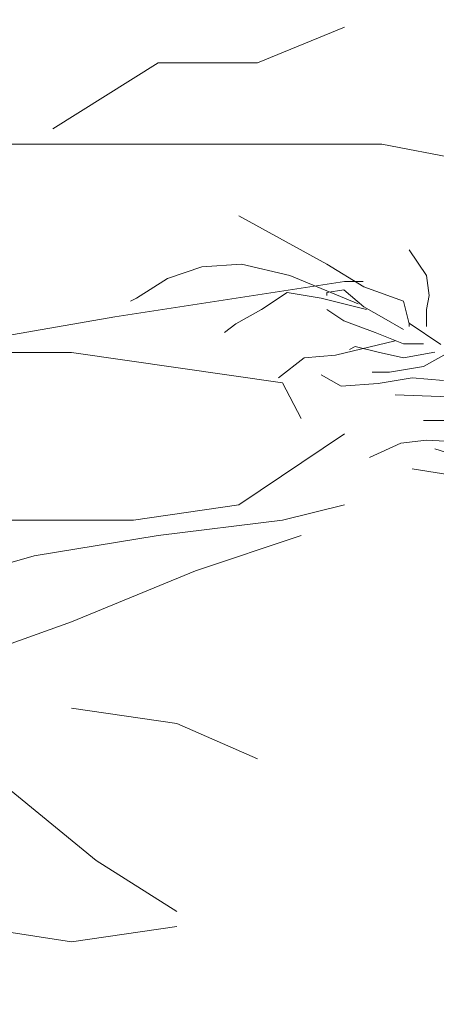
# Model space of a CAD drawing. Units: millimetres. Extents: x 595116 to 630915, y 909473 to 920225.
# Tile 21 of 134: x 629595.851 to 629599.598, y 919171.91 to 919180.767. Entities that reach past the tile are written whole.
import ezdxf

# ---------------------------------------------------------------- set-up
doc = ezdxf.new("R2010")
doc.units = ezdxf.units.MM
doc.layers.add('Dimension', color=3, linetype='Continuous', lineweight=18)
doc.layers.add('L-PLNT', color=85, linetype='Continuous', lineweight=13)
doc.styles.get("Standard").update_dxf_attribs({"font": 'arial.ttf'})
doc.dimstyles.new('ISO-25', dxfattribs={"dimtxt": 9, "dimasz": 6, "dimexe": 1.25, "dimexo": 0.625, "dimtad": 1, "dimlunit": 4, "dimtxsty": 'Standard', "dimcen": 2.5, "dimadec": 0, "dimazin": 0, "dimtfac": 1, "dimtmove": 0, "dimatfit": 3, "dimfxl": 1, "dimarcsym": 0})

# ---------------------------------------------------------------- blocks, each defined once
blk = doc.blocks.new('A$C143125F4')
for p, q in [((4.78124, 2.3788), (4.85783, 2.41016)), ((4.60071, 2.32057), (4.69371, 2.3788)), ((4.69371, 2.3788), (4.78124, 2.3788)), ((4.32719, 2.30713), (4.89065, 2.30713)), ((4.89065, 2.30713), (4.98365, 2.28921)), ((4.65542, 2.15481), (4.85783, 2.18617)), ((4.85783, 2.18617), (4.87424, 2.18617)), ((4.47489, 2.12345), (4.65542, 2.15481)), ((4.50771, 2.12345), (4.61712, 2.12345)), ((4.61712, 2.12345), (4.80312, 2.09657)), ((4.80312, 2.09657), (4.81953, 2.06521)), ((4.85783, 2.05177), (4.76483, 1.98906)), ((4.76483, 1.98906), (4.67183, 1.97562)), ((4.80312, 1.97562), (4.85783, 1.98906)), ((4.67183, 1.97562), (4.20136, 1.97562)), ((4.69371, 1.96218), (4.80312, 1.97562)), ((4.5843, 1.94426), (4.69371, 1.96218)), ((4.81953, 1.96218), (4.72653, 1.93082)), ((4.4913, 1.91738), (4.5843, 1.94426)), ((4.72653, 1.93082), (4.61712, 1.88602)), ((4.61712, 1.88602), (4.5296, 1.85466)), ((4.61712, 1.80986), (4.71012, 1.79642)), ((4.71012, 1.79642), (4.78124, 1.76506)), ((4.54601, 1.75162), (4.63901, 1.67547)), ((4.63901, 1.67547), (4.71012, 1.63067)), ((4.5296, 1.61723), (4.61712, 1.60379)), ((4.61712, 1.60379), (4.71012, 1.61723))]:
    blk.add_line(p, q)
blk = doc.blocks.new('A$C4FB75ABC')
for p, q in [((0.4999, 4.2779), (0.7111, 4.1621)), ((0.9087, 4.1962), (0.9496, 4.1349)), ((0.4114, 4.1553), (0.3296, 4.1281)), ((0.5068, 4.1621), (0.4114, 4.1553)), ((0.6226, 4.1349), (0.5068, 4.1621)), ((0.7111, 4.1621), (0.7997, 4.1076)), ((0.7861, 4.0668), (0.6226, 4.1349)), ((0.9496, 4.1349), (0.9564, 4.0872)), ((0.3296, 4.1281), (0.2547, 4.0804)), ((0.7997, 4.1076), (0.8951, 4.0736)), ((0.6158, 4.094), (0.5544, 4.0532)), ((0.6975, 4.0804), (0.6158, 4.094)), ((0.752, 4.1008), (0.7111, 4.094)), ((0.7111, 4.094), (0.7111, 4.0872)), ((0.7997, 4.06), (0.752, 4.1008)), ((0.9564, 4.0872), (0.9496, 4.0532)), ((0.2547, 4.0804), (0.241, 4.0736)), ((0.8065, 4.0532), (0.6975, 4.0804)), ((0.8474, 4.0327), (0.7997, 4.06)), ((0.8951, 4.0736), (0.9087, 4.0191)), ((0.5544, 4.0532), (0.4931, 4.0191)), ((0.7111, 4.0532), (0.752, 4.0259)), ((0.9496, 4.0532), (0.9496, 4.0123)), ((0.4931, 4.0191), (0.4659, 3.9987)), ((0.752, 4.0259), (0.827, 3.9987)), ((0.8951, 4.0055), (0.8474, 4.0327)), ((0.9842, 3.9699), (0.9085, 4.0207)), ((0.9087, 4.0191), (0.9087, 4.0123)), ((0.827, 3.9987), (0.8951, 3.9715)), ((0.8746, 3.9783), (0.7316, 3.9442)), ((0.7793, 3.9647), (0.7656, 3.9578)), ((0.8338, 3.951), (0.7793, 3.9647)), ((0.8951, 3.9715), (0.9428, 3.9715)), ((0.7316, 3.9442), (0.6566, 3.9374)), ((0.8951, 3.9374), (0.8338, 3.951)), ((0.97, 3.951), (0.8951, 3.9374)), ((1.0041, 3.951), (0.9428, 3.917)), ((0.6566, 3.9374), (0.5953, 3.8897)), ((0.7452, 3.8693), (0.6975, 3.8966)), ((0.861, 3.9034), (0.8201, 3.9034)), ((0.9428, 3.917), (0.861, 3.9034)), ((0.8338, 3.8761), (0.7452, 3.8693)), ((0.9155, 3.8897), (0.8338, 3.8761)), ((0.9905, 3.8829), (0.9155, 3.8897)), ((0.8746, 3.8489), (1.0518, 3.8421)), ((0.9428, 3.7876), (1.0382, 3.7876)), ((0.8133, 3.6991), (0.8883, 3.7331)), ((0.8883, 3.7331), (0.9496, 3.7399)), ((0.9496, 3.7399), (1.079, 3.7331)), ((0.97, 3.7195), (1.1403, 3.665)), ((0.9155, 3.6718), (1.1267, 3.6378))]:
    blk.add_line(p, q)
blk = doc.blocks.new('*D216')
at = {"layer": 'Defpoints', "color": 0, "transparency": 16777216}
for p in [(629743.5408, 919411.9276), (629505.0408, 919411.8279), (629743.5408, 918832.3776)]:
    blk.add_point(p, dxfattribs=at)
at = {"layer": 'Dimension', "color": 0, "lineweight": -2, "transparency": 16777216}
for p, q in [((629743.5408, 919411.3026), (629743.5408, 918831.1276)), ((629505.0408, 919411.2029), (629505.0408, 918831.1276)), ((629511.0408, 918832.3776), (629737.5408, 918832.3776))]:
    blk.add_line(p, q, dxfattribs=at)
at = {"layer": 'Dimension', "color": 0, "transparency": 16777216}
for points in [[(629511.0408, 918833.3776), (629511.0408, 918831.3776), (629505.0408, 918832.3776)], [(629737.5408, 918833.3776), (629737.5408, 918831.3776), (629743.5408, 918832.3776)]]:
    blk.add_solid(points, dxfattribs=at)
at = {"layer": 'Dimension', "color": 0, "transparency": 16777216, "insert": (629624.2908, 918837.656), "char_height": 9, "attachment_point": 5}
blk.add_mtext('19\'-10 1/2"', dxfattribs=at)

msp = doc.modelspace()

# ---------------------------------------------------------------- block references
at = {"layer": 'L-PLNT'}
for name, p, xscale, yscale, zscale in [('A$C143125F4', (629549.214, 919156.1107), 10.20167662382051, 10.20167662382051, 10.20167662382051), ('A$C4FB75ABC', (629595.9442, 919162.9458), 3.753413438031968, 3.753413438031968, 3.753413438031968)]:
    msp.add_blockref(name, p, dxfattribs=dict(at, xscale=xscale, yscale=yscale, zscale=zscale))

# ---------------------------------------------------------------- dimensions: what is measured, and where the dimension line sits
at = {"layer": 'Dimension'}
dim = msp.add_linear_dim(base=(629743.5408, 918832.3776), p1=(629505.0408, 919411.8279), p2=(629743.5408, 919411.9276), dimstyle='ISO-25', override={"dimdec": 1, "dimlfac": 1, "dimrnd": 0, "dimzin": 1, "dimdsep": 46, "dimlunit": 4, "dimfrac": 2}, dxfattribs=at)
dim.commit()
dim.dimension.update_dxf_attribs({"geometry": '*D216', "text_midpoint": (629624.2908, 918837.656)})

doc.saveas('drawing.dxf')
